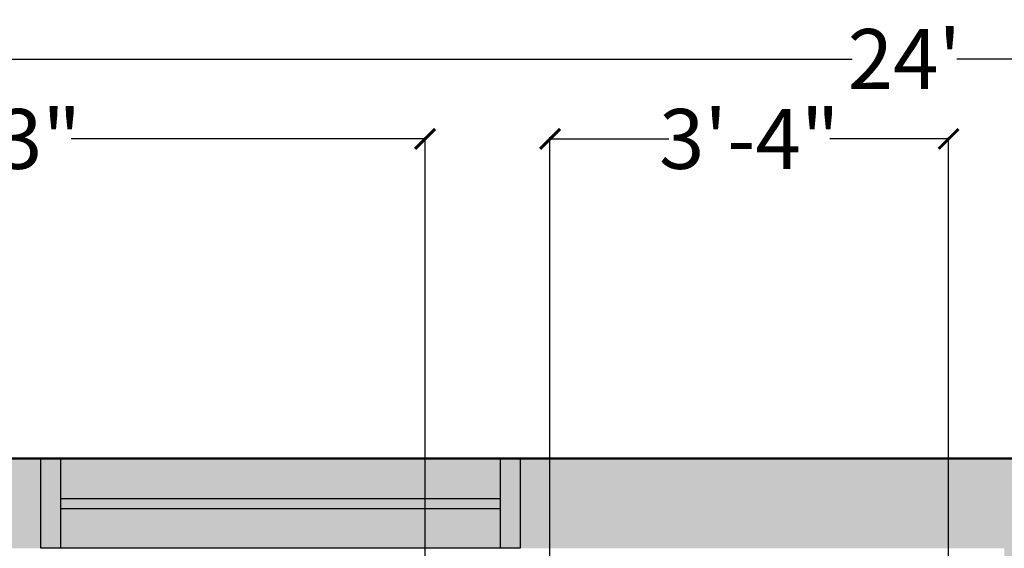
# Model space of a CAD drawing. Units: inches. Extents: x 528 to 2620, y -1066 to 798.
# Tile 31 of 41: x 1112 to 1211, y 710 to 763. Entities that reach past the tile are written whole.
import ezdxf

# ---------------------------------------------------------------- set-up
doc = ezdxf.new("R2010")
doc.units = ezdxf.units.IN
doc.header["$MEASUREMENT"] = 0
for name, color, linetype, lineweight in [('A-ANNO-DIMS', 2, 'Continuous', 18), ('A-GLAZ', 3, 'Continuous', 25), ('A-WALL', 7, 'Continuous', 50), ('A-WALL-PATT', 8, 'Continuous', 13)]:
    doc.layers.add(name, color=color, linetype=linetype, lineweight=lineweight)
doc.styles.get("Standard").update_dxf_attribs({"font": 'arial.ttf'})
doc.dimstyles.get("Standard").update_dxf_attribs({"dimtxt": 6, "dimasz": 2, "dimexe": 0.18, "dimexo": 0.0625, "dimgap": 0.09, "dimtad": 0, "dimtih": 1, "dimtoh": 1, "dimdec": 1, "dimzin": 0, "dimdsep": 46, "dimlunit": 3, "dimtxsty": 'Standard', "dimblk": 'ARCHTICK', "dimcen": 0.09, "dimadec": 0, "dimazin": 0, "dimtfac": 1, "dimtdec": 1, "dimtofl": 0, "dimtmove": 0, "dimatfit": 3, "dimfxl": 1, "dimtolj": 1, "dimtzin": 0, "dimarcsym": 0})

# ---------------------------------------------------------------- blocks, each defined once
blk = doc.blocks.new('_ArchTick')
at = {"color": 0, "linetype": 'ByBlock', "const_width": 0.15}
blk.add_lwpolyline([(-0.5, -0.5), (0.5, 0.5)], dxfattribs=at)
blk = doc.blocks.new('*D18')
at = {"layer": 'A-ANNO-DIMS', "color": 0, "lineweight": -2, "transparency": 16777216}
for p, q in [((1056.996, 718.985), (1056.996, 759.108)), ((1056.996, 758.928), (1195.764, 758.928)), ((1344.996, 758.928), (1206.229, 758.928)), ((1344.996, 718.985), (1344.996, 759.108))]:
    blk.add_line(p, q, dxfattribs=at)
at = {"layer": 'Defpoints', "color": 0, "transparency": 16777216}
for p in [(1344.996, 758.928), (1056.996, 718.922), (1344.996, 718.922)]:
    blk.add_point(p, dxfattribs=at)
at = {"layer": 'A-ANNO-DIMS', "color": 0, "lineweight": -2, "transparency": 16777216, "xscale": 2, "yscale": 2, "zscale": 2, "rotation": 180}
blk.add_blockref('_ArchTick', (1056.996, 758.928), dxfattribs=at)
at = {"layer": 'A-ANNO-DIMS', "color": 0, "lineweight": -2, "transparency": 16777216, "xscale": 2, "yscale": 2, "zscale": 2}
blk.add_blockref('_ArchTick', (1344.996, 758.928), dxfattribs=at)
at = {"layer": 'A-ANNO-DIMS', "color": 0, "transparency": 16777216, "insert": (1200.996, 758.928), "char_height": 6, "attachment_point": 5}
blk.add_mtext("\\A1;24'", dxfattribs=at)
blk = doc.blocks.new('WIN-1200')
for p, q in [((677.559, 718.922), (725.559, 718.922)), ((677.559, 709.922), (677.559, 718.922)), ((679.559, 709.922), (679.559, 718.922)), ((723.559, 718.922), (723.559, 709.922)), ((725.559, 718.922), (725.559, 709.922)), ((679.559, 714.922), (723.559, 714.922)), ((679.559, 713.922), (723.559, 713.922)), ((725.559, 709.922), (677.559, 709.922))]:
    blk.add_line(p, q)
blk = doc.blocks.new('*D58')
at = {"layer": 'A-ANNO-DIMS', "color": 0, "lineweight": -2, "transparency": 16777216}
for p, q in [((1165.496, 577.985), (1165.496, 751.102)), ((1165.496, 750.922), (1177.395, 750.922)), ((1205.418, 750.922), (1193.52, 750.922)), ((1205.418, 577.985), (1205.418, 751.102))]:
    blk.add_line(p, q, dxfattribs=at)
at = {"layer": 'Defpoints', "color": 0, "transparency": 16777216}
for p in [(1205.418, 750.922), (1165.496, 577.922), (1205.418, 577.922)]:
    blk.add_point(p, dxfattribs=at)
at = {"layer": 'A-ANNO-DIMS', "color": 0, "lineweight": -2, "transparency": 16777216, "xscale": 2, "yscale": 2, "zscale": 2, "rotation": 180}
blk.add_blockref('_ArchTick', (1165.496, 750.922), dxfattribs=at)
at = {"layer": 'A-ANNO-DIMS', "color": 0, "lineweight": -2, "transparency": 16777216, "xscale": 2, "yscale": 2, "zscale": 2}
blk.add_blockref('_ArchTick', (1205.418, 750.922), dxfattribs=at)
at = {"layer": 'A-ANNO-DIMS', "color": 0, "transparency": 16777216, "insert": (1185.457, 750.922), "char_height": 6, "attachment_point": 5}
blk.add_mtext('\\A1;3\'-4"', dxfattribs=at)
blk = doc.blocks.new('*D66')
at = {"layer": 'A-ANNO-DIMS', "color": 0, "lineweight": -2, "transparency": 16777216}
for p, q in [((1065.996, 400.485), (1065.996, 751.102)), ((1065.996, 750.922), (1101.456, 750.922)), ((1152.996, 750.922), (1117.537, 750.922)), ((1152.996, 400.485), (1152.996, 751.102))]:
    blk.add_line(p, q, dxfattribs=at)
at = {"layer": 'Defpoints', "color": 0, "transparency": 16777216}
for p in [(1152.996, 750.922), (1065.996, 400.422), (1152.996, 400.422)]:
    blk.add_point(p, dxfattribs=at)
at = {"layer": 'A-ANNO-DIMS', "color": 0, "lineweight": -2, "transparency": 16777216, "xscale": 2, "yscale": 2, "zscale": 2, "rotation": 180}
blk.add_blockref('_ArchTick', (1065.996, 750.922), dxfattribs=at)
at = {"layer": 'A-ANNO-DIMS', "color": 0, "lineweight": -2, "transparency": 16777216, "xscale": 2, "yscale": 2, "zscale": 2}
blk.add_blockref('_ArchTick', (1152.996, 750.922), dxfattribs=at)
at = {"layer": 'A-ANNO-DIMS', "color": 0, "transparency": 16777216, "insert": (1109.496, 750.922), "char_height": 6, "attachment_point": 5}
blk.add_mtext('\\A1;7\'-3"', dxfattribs=at)

msp = doc.modelspace()

# ---------------------------------------------------------------- hatches: boundary and pattern name
at = {"layer": 'A-WALL-PATT', "transparency": 33554521}
h = msp.add_hatch(color=256, dxfattribs=at)
h.dxf.hatch_style = 1
h.paths.add_polyline_path([(1065.996, 709.922), (1114.496, 709.922), (1114.496, 718.922), (1056.996, 718.922), (1056.996, 667.922), (1065.996, 667.922)])
h.paths.add_polyline_path([(1227.496, 718.922), (1162.496, 718.922), (1162.496, 709.922), (1210.996, 709.922), (1210.996, 577.922), (1205.418, 577.922), (1205.496, 573.422), (1210.996, 573.422), (1210.996, 567.422), (1215.496, 567.422), (1215.496, 669.422), (1267.996, 669.422), (1267.996, 675.922), (1263.496, 675.922), (1263.496, 673.922), (1215.496, 673.922), (1215.496, 709.922), (1227.496, 709.922)])
h.paths.add_polyline_path([(1344.996, 718.922), (1315.996, 718.922), (1315.996, 709.922), (1335.996, 709.922), (1335.996, 641.672), (1344.996, 641.672)])
h.paths.add_polyline_path([(1065.996, 619.922), (1056.996, 619.922), (1056.996, 561.422), (1065.996, 561.422), (1065.996, 573.422), (1160.996, 573.422), (1160.996, 569.422), (1165.496, 569.422), (1165.496, 577.922), (1065.996, 577.922)])
h.paths.add_polyline_path([(1215.996, 391.422), (1215.996, 400.422), (1206.996, 400.422), (1200.996, 400.422), (1200.996, 397.422), (1200.996, 391.422), (1206.996, 391.422), (1206.996, 268.922), (1251.996, 268.922), (1251.996, 277.922), (1215.996, 277.922), (1215.996, 359.767)])
h.paths.add_polyline_path([(1344.996, 395.922), (1335.996, 395.922), (1287.996, 395.922), (1287.996, 391.422), (1335.996, 391.422), (1335.996, 277.922), (1299.996, 277.922), (1299.996, 268.922), (1344.996, 268.922)])
h.paths.add_polyline_path([(1344.996, 593.672), (1335.996, 593.672), (1335.996, 525.422), (1215.496, 525.422), (1215.496, 527.172), (1210.996, 527.172), (1210.996, 520.922), (1335.996, 520.922), (1335.996, 443.922), (1344.996, 443.922)])
h.paths.add_polyline_path([(1065.996, 520.922), (1165.496, 520.922), (1165.496, 545.422), (1160.996, 545.422), (1160.996, 525.422), (1065.996, 525.422), (1065.996, 537.422), (1056.996, 537.422), (1056.996, 484.672), (1065.996, 484.672)])
h.paths.add_polyline_path([(1065.996, 436.672), (1056.996, 436.672), (1056.996, 391.422), (1085.496, 391.422), (1085.496, 400.422), (1065.996, 400.422)])
h.paths.add_polyline_path([(1152.996, 397.422), (1152.996, 400.422), (1133.496, 400.422), (1133.496, 391.422), (1152.996, 391.422)])
at = {"layer": 'A-WALL-PATT', "transparency": 33554681}
h = msp.add_hatch(color=256, dxfattribs=at)
h.dxf.hatch_style = 1
h.paths.add_polyline_path([(1061.996, 665.922), (1060.996, 665.922), (1060.996, 621.922), (1061.996, 621.922)])
h.paths.add_polyline_path([(1065.996, 667.922), (1056.996, 667.922), (1056.996, 665.922), (1065.996, 665.922)])
h.paths.add_polyline_path([(1065.996, 621.922), (1056.996, 621.922), (1056.996, 619.922), (1065.996, 619.922)])
h.paths.add_polyline_path([(1160.496, 714.922), (1116.496, 714.922), (1116.496, 713.922), (1160.496, 713.922)])
h.paths.add_polyline_path([(1162.496, 718.922), (1160.496, 718.922), (1160.496, 709.922), (1162.496, 709.922)])
h.paths.add_polyline_path([(1116.496, 718.922), (1114.496, 718.922), (1114.496, 709.922), (1116.496, 709.922)])
h.paths.add_polyline_path([(1251.496, 714.922), (1227.496, 714.922), (1227.496, 713.922), (1251.496, 713.922)])
h.paths.add_polyline_path([(1313.996, 714.922), (1269.996, 714.922), (1269.996, 713.922), (1313.996, 713.922)])
h.paths.add_polyline_path([(1315.996, 718.922), (1313.996, 718.922), (1313.996, 709.922), (1315.996, 709.922)])
h.paths.add_polyline_path([(1269.996, 718.922), (1267.996, 718.922), (1267.996, 709.922), (1269.996, 709.922)])
h.paths.add_polyline_path([(1087.496, 400.422), (1085.496, 400.422), (1085.496, 391.422), (1087.496, 391.422)])
h.paths.add_polyline_path([(1131.496, 396.422), (1087.496, 396.422), (1087.496, 395.422), (1131.496, 395.422)])
h.paths.add_polyline_path([(1133.496, 400.422), (1131.496, 400.422), (1131.496, 391.422), (1133.496, 391.422)])
h.paths.add_polyline_path([(1065.996, 438.672), (1056.996, 438.672), (1056.996, 436.672), (1065.996, 436.672)])
h.paths.add_polyline_path([(1065.996, 484.672), (1056.996, 484.672), (1056.996, 482.672), (1065.996, 482.672)])
h.paths.add_polyline_path([(1061.996, 482.672), (1060.996, 482.672), (1060.996, 438.672), (1061.996, 438.672)])
h = msp.add_hatch(color=256, dxfattribs=at)
h.dxf.hatch_style = 1
h.paths.add_polyline_path([(1065.996, 665.922), (1061.996, 665.922), (1061.996, 621.922), (1065.996, 621.922)])
h.paths.add_polyline_path([(1060.996, 665.922), (1056.996, 665.922), (1056.996, 621.922), (1060.996, 621.922)])
h.paths.add_polyline_path([(1160.496, 713.922), (1116.496, 713.922), (1116.496, 709.922), (1160.496, 709.922)])
h.paths.add_polyline_path([(1160.496, 718.922), (1116.496, 718.922), (1116.496, 714.922), (1160.496, 714.922)])
h.paths.add_polyline_path([(1251.496, 713.922), (1227.496, 713.922), (1227.496, 709.922), (1251.496, 709.922)])
h.paths.add_polyline_path([(1251.496, 718.922), (1227.496, 718.922), (1227.496, 714.922), (1251.496, 714.922)])
h.paths.add_polyline_path([(1313.996, 713.922), (1269.996, 713.922), (1269.996, 709.922), (1313.996, 709.922)])
h.paths.add_polyline_path([(1313.996, 718.922), (1269.996, 718.922), (1269.996, 714.922), (1313.996, 714.922)])
h.paths.add_polyline_path([(1344.996, 639.672), (1340.996, 639.672), (1340.996, 595.672), (1344.996, 595.672)])
h.paths.add_polyline_path([(1339.996, 639.672), (1335.996, 639.672), (1335.996, 595.672), (1339.996, 595.672)])
h.paths.add_polyline_path([(1344.996, 441.922), (1340.996, 441.922), (1340.996, 397.922), (1344.996, 397.922)])
h.paths.add_polyline_path([(1339.996, 441.922), (1335.996, 441.922), (1335.996, 397.922), (1339.996, 397.922)])
h.paths.add_polyline_path([(1297.996, 272.922), (1253.996, 272.922), (1253.996, 268.922), (1297.996, 268.922)])
h.paths.add_polyline_path([(1297.996, 277.922), (1253.996, 277.922), (1253.996, 273.922), (1297.996, 273.922)])
h.paths.add_polyline_path([(1131.496, 395.422), (1087.496, 395.422), (1087.496, 391.422), (1131.496, 391.422)])
h.paths.add_polyline_path([(1131.496, 400.422), (1087.496, 400.422), (1087.496, 396.422), (1131.496, 396.422)])
h.paths.add_polyline_path([(1065.996, 482.672), (1061.996, 482.672), (1061.996, 438.672), (1065.996, 438.672)])
h.paths.add_polyline_path([(1060.996, 482.672), (1056.996, 482.672), (1056.996, 438.672), (1060.996, 438.672)])
h.paths.add_polyline_path([(1065.996, 561.422), (1061.996, 561.422), (1061.996, 537.422), (1065.996, 537.422)])
h.paths.add_polyline_path([(1060.996, 561.422), (1056.996, 561.422), (1056.996, 537.422), (1060.996, 537.422)])

# ---------------------------------------------------------------- linework, layer by layer
at = {"layer": 'A-WALL'}
msp.add_line((1344.996, 718.922), (1056.996, 718.922), dxfattribs=at)

# ---------------------------------------------------------------- block references
at = {"layer": 'A-GLAZ'}
msp.add_blockref('WIN-1200', (436.937, 0), dxfattribs=at)

# ---------------------------------------------------------------- dimensions: what is measured, and where the dimension line sits
at = {"layer": 'A-ANNO-DIMS'}
for base, p1, p2, override, picture, middle in [((1344.996, 758.928), (1056.996, 718.922), (1344.996, 718.922), {"dimclrd": 0, "dimclre": 0, "dimclrt": 0}, '*D18', (1200.996, 758.928)), ((1152.996, 750.922), (1065.996, 400.422), (1152.996, 400.422), {"dimdec": 1, "dimlfac": 1, "dimrnd": 0, "dimzin": 1, "dimdsep": 46, "dimlunit": 4, "dimfrac": 2}, '*D66', (1109.496, 750.922)), ((1205.418, 750.922), (1165.496, 577.922), (1205.418, 577.922), {"dimdec": 1, "dimlfac": 1, "dimrnd": 0, "dimzin": 1, "dimdsep": 46, "dimlunit": 4, "dimfrac": 2}, '*D58', (1185.457, 750.922))]:
    dim = msp.add_linear_dim(base=base, p1=p1, p2=p2, dimstyle='Standard', override=override, dxfattribs=at)
    dim.commit()
    dim.dimension.update_dxf_attribs({"geometry": picture, "text_midpoint": middle})

doc.saveas('drawing.dxf')
